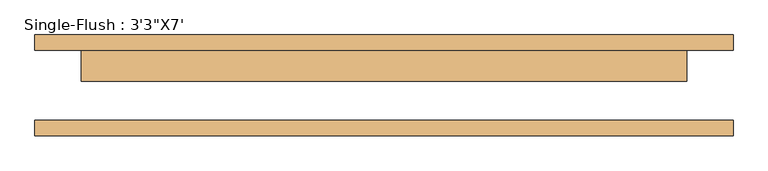
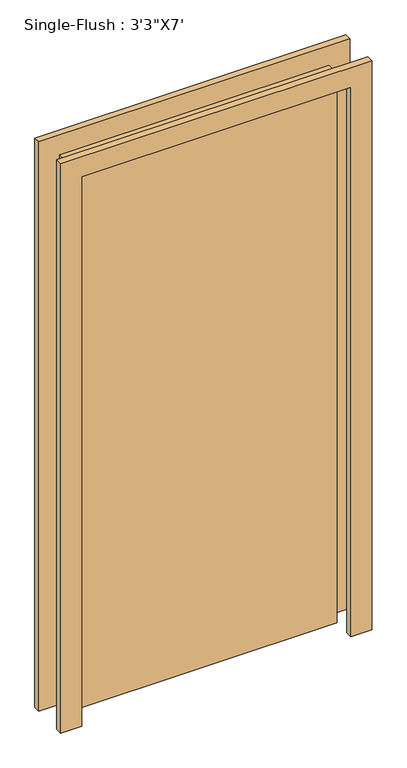
"""IFC4 building model written with IfcOpenShell, lengths in millimetres: door geometry."""

from ifc_helpers import new_model, si_unit, frame, origin, origin_with_axes, place, context, project, spatial, polyline, outline, extrude, source, transform, mapped, element, save


def door_0217d254(model_context):
    return source(origin(), model_context, "Body", "SweptSolid", [
        extrude(outline(polyline([(2209.8, -571.5), (0.0, -571.5), (0.0, -495.3), (2133.6, -495.3), (2133.6, 495.3), (0.0, 495.3), (0.0, 571.5), (2209.8, 571.5), (2209.8, -571.5)])), frame((0.0, 57.15, 0.0), z_axis=(0.0, 1.0, 0.0), x_axis=(0.0, 0.0, 1.0)), (0.0, 0.0, 1.0), 25.4),
        extrude(outline(polyline([(2209.8, 571.5), (2209.8, -571.5), (0.0, -571.5), (0.0, -495.3), (2133.6, -495.3), (2133.6, 495.3), (0.0, 495.3), (0.0, 571.5), (2209.8, 571.5)])), frame((0.0, -82.55, 0.0), z_axis=(0.0, 1.0, 0.0), x_axis=(0.0, 0.0, 1.0)), (0.0, 0.0, 1.0), 25.4),
        extrude(outline(polyline([(495.3, 6.35), (-495.3, 6.35), (-495.3, 57.15), (495.3, 57.15), (495.3, 6.35)])), origin_with_axes(), (0.0, 0.0, 1.0), 2133.6),
    ])


if __name__ == "__main__":
    model = new_model("IFC4")
    model_context = context("Model", 3, world=origin())
    ifc_project = project(units=[si_unit("LENGTHUNIT", "METRE", prefix="MILLI")], contexts=[model_context])
    site = spatial("IfcSite", under=ifc_project)
    building = spatial("IfcBuilding", under=site)
    placement = place(None, origin())
    door_shape = door_0217d254(model_context)
    element("IfcDoor", 1, ObjectType="Single-Flush : 3'3\"X7'", at=placement, inside=building, context=model_context, shape_type="MappedRepresentation", body=[
        mapped(door_shape, transform((0.0, 0.0, 0.0), x_axis=(1.0, 0.0, 0.0), y_axis=(0.0, 1.0, 0.0), z_axis=(0.0, 0.0, 1.0))),
    ])
    save(model, "model.ifc")

# Revit data of these elements
# Type "Single-Flush : 3'3\"X7'"
#   Type Mark = "11"
#   Construction Type Id = "MDOOR"
#   Assembly Code = "C1020"
#   Analytic Construction = "Metal"
#   Thickness = 0' - 2"
#   Heat Transfer Coefficient (U) = 0.651978 BTU/(h·ft²·°F)
#   Height = 7' - 0"
#   Trim Projection Ext = 0' - 1"
#   Trim Projection Int = 0' - 1"
#   Trim Width = 0' - 3"
#   Width = 3' - 3"
#   Define Thermal Properties by = 1
#   Door Material = Door - Panel
#   Frame Material = Door - Frame
#   Visual Light Transmittance = 0
#   Solar Heat Gain Coefficient = 0
#   Function = (empty or 0)
#   Wall Closure = (empty or 0)
# Element 1 (IfcDoor, "Single-Flush : 3'3\"X7'")
#   Materials on its faces: "Door - Frame", "Door - Panel"
# Materials
#   "Door - Panel": class "Wood", colour RGB 210 159 95, transparency 0, Cost = 0
#   "Door - Frame": colour RGB 118 70 51, transparency 0, Cost = 0
